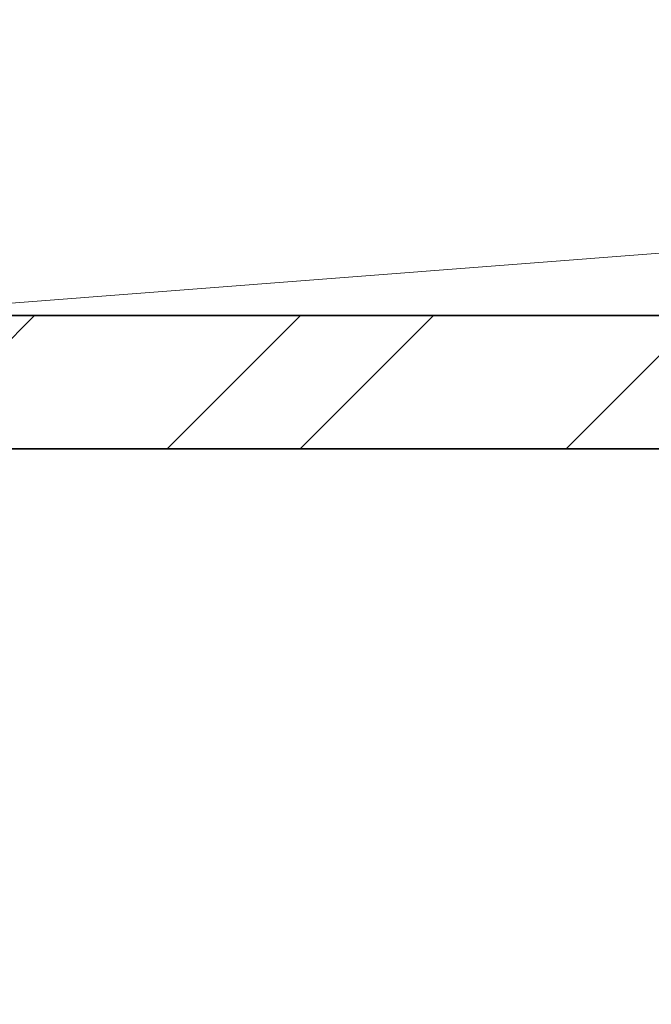
# Model space of a CAD drawing. Units: inches. Extents: x 1885 to 2748, y 783 to 2421.
# Tile 36 of 117: x 2013 to 2034, y 1501 to 1534. Entities that reach past the tile are written whole.
import ezdxf

# ---------------------------------------------------------------- set-up
doc = ezdxf.new("R2010")
doc.units = ezdxf.units.IN
doc.layers.add('A-FLOR-OPEN', color=8, linetype='Continuous', lineweight=13)
doc.layers.add('A-WALL', color=7, linetype='Continuous', lineweight=35)
doc.layers.add('A-WALL-PATT', color=85, linetype='Continuous', lineweight=13, true_color=0x58ba48)

msp = doc.modelspace()

# ---------------------------------------------------------------- hatches: boundary and pattern name
at = {"layer": 'A-WALL-PATT'}
h = msp.add_hatch(dxfattribs=at)
h.set_pattern_fill('ANSI32', color=256)
h.paths.add_polyline_path([(2007.772, 2318.006), (1980.774, 2318.006), (1980.774, 2281.215), (1985.274, 2281.215), (1985.274, 2313.506), (2007.772, 2313.506), (2007.772, 2315.756)])
h.paths.add_polyline_path([(2094.324, 2318.006), (2067.772, 2318.006), (2067.772, 2313.506), (2094.324, 2313.506), (2094.324, 2315.756)])
h.paths.add_polyline_path([(2131.367, 2315.756), (2131.367, 2318.006), (2131.189, 2318.006), (2112.609, 2318.006), (2112.609, 2313.506), (2117.274, 2313.506), (2117.274, 2255.201), (2121.774, 2255.201), (2121.774, 2313.506), (2131.367, 2313.506)])
h.paths.add_polyline_path([(2190.512, 2318.006), (2155.367, 2318.006), (2155.367, 2313.506), (2169.774, 2313.506), (2169.774, 2229.506), (2121.774, 2229.506), (2121.774, 2233.451), (2119.524, 2233.451), (2117.274, 2233.451), (2117.274, 2201.101), (2121.774, 2201.101), (2121.774, 2225.006), (2169.774, 2225.006), (2169.774, 2165.006), (2306.274, 2165.006), (2306.274, 2066.006), (2310.774, 2066.006), (2344.274, 2066.006), (2486.274, 2066.006), (2486.274, 1886.006), (2483.02, 1886.006), (2483.02, 1881.506), (2486.274, 1881.506), (2486.274, 1880.678), (2490.774, 1880.678), (2490.774, 2070.506), (2344.274, 2070.506), (2310.774, 2070.506), (2310.774, 2165.006), (2310.774, 2173.636), (2308.524, 2173.636), (2306.274, 2173.636), (2306.274, 2169.506), (2174.274, 2169.506), (2174.274, 2313.506), (2190.512, 2313.506), (2190.512, 2315.756)])
h.paths.add_polyline_path([(1985.274, 2221.215), (1980.774, 2221.215), (1980.774, 2165.006), (1992.774, 2165.006), (1992.774, 2141.927), (1997.274, 2141.927), (1997.274, 2165.006), (2117.274, 2165.006), (2117.274, 2163.126), (2121.774, 2163.126), (2121.774, 2172.734), (2119.524, 2172.734), (2117.274, 2172.734), (2117.274, 2169.506), (1985.274, 2169.506)])
h.paths.add_polyline_path([(1997.274, 2105.927), (1992.774, 2105.927), (1992.774, 2070.506), (2016.774, 2070.506), (2016.774, 2059.123), (2019.024, 2059.123), (2021.274, 2059.123), (2021.274, 2070.506), (2117.274, 2070.506), (2117.274, 2022.506), (2114.423, 2022.506), (2114.423, 2018.006), (2123.627, 2018.006), (2123.627, 2020.256), (2123.627, 2022.506), (2121.774, 2022.506), (2121.774, 2142.587), (2119.524, 2142.587), (2117.274, 2142.587), (2117.274, 2075.006), (1997.274, 2075.006)])
h.paths.add_polyline_path([(2092.029, 2020.256), (2092.029, 2022.506), (2021.274, 2022.506), (2021.274, 2035.123), (2016.774, 2035.123), (2016.774, 2018.006), (2016.774, 1978.784), (2021.274, 1978.784), (2021.274, 2018.006), (2092.029, 2018.006)])
h.paths.add_polyline_path([(2260.938, 2022.506), (2153.105, 2022.506), (2153.105, 2020.256), (2153.105, 2018.006), (2155.274, 2018.006), (2155.274, 1886.006), (2107.629, 1886.006), (2107.629, 1881.506), (2182.911, 1881.506), (2182.911, 1883.756), (2182.911, 1886.006), (2159.774, 1886.006), (2159.774, 2018.006), (2260.938, 2018.006), (2260.938, 2020.256)])
h.paths.add_polyline_path([(2047.629, 1883.756), (2047.629, 1886.006), (2021.274, 1886.006), (2021.274, 1918.784), (2019.024, 1918.784), (2016.774, 1918.784), (2016.774, 1881.506), (2047.629, 1881.506)])
h.paths.add_polyline_path([(2306.361, 1883.756), (2306.361, 1886.006), (2296.274, 1886.006), (2296.274, 1982.006), (2316.535, 1982.006), (2316.535, 1984.256), (2316.535, 1986.506), (2296.274, 1986.506), (2296.274, 2022.506), (2289.276, 2022.506), (2289.276, 2018.006), (2291.774, 2018.006), (2291.774, 1886.006), (2242.911, 1886.006), (2242.911, 1881.506), (2306.361, 1881.506)], flags=17)
h.paths.add_polyline_path([(1985.274, 1843.006), (2021.6, 1843.006), (2021.534, 1845.441), (2021.477, 1847.506), (1980.774, 1847.506), (1980.774, 1809.446), (1985.274, 1809.446)])
h.paths.add_polyline_path([(2131.482, 1845.256), (2131.482, 1847.506), (2081.534, 1847.506), (2081.534, 1843.006), (2117.274, 1843.006), (2117.274, 1784.147), (2119.524, 1784.147), (2121.774, 1784.147), (2121.774, 1843.006), (2131.482, 1843.006)])
h.paths.add_polyline_path([(2203.886, 1847.506), (2155.482, 1847.506), (2155.482, 1843.006), (2169.774, 1843.006), (2169.774, 1759.006), (2121.774, 1759.006), (2121.774, 1761.457), (2117.274, 1761.457), (2117.274, 1730.429), (2121.774, 1730.429), (2121.774, 1754.506), (2177.421, 1754.506), (2177.421, 1756.756), (2177.421, 1759.006), (2174.274, 1759.006), (2174.274, 1843.006), (2203.886, 1843.006)])
h.paths.add_polyline_path([(2335.554, 1845.256), (2335.554, 1847.506), (2239.886, 1847.506), (2239.886, 1843.006), (2306.274, 1843.006), (2306.274, 1759.006), (2199.486, 1759.006), (2199.486, 1754.506), (2310.774, 1754.506), (2310.774, 1843.006), (2335.554, 1843.006)])
h.paths.add_polyline_path([(2348.774, 2022.506), (2344.274, 2022.506), (2344.274, 1986.506), (2341.681, 1986.506), (2341.681, 1982.006), (2344.274, 1982.006), (2344.274, 1886.006), (2330.361, 1886.006), (2330.361, 1881.506), (2361.627, 1881.506), (2361.627, 1883.756), (2361.627, 1886.006), (2348.774, 1886.006)], flags=17)
h.paths.add_polyline_path([(2283.251, 2315.756), (2283.251, 2318.006), (2238.512, 2318.006), (2238.512, 2313.506), (2283.251, 2313.506)], flags=17)
h.paths.add_polyline_path([(2363.274, 2348.006), (2388.677, 2348.006), (2388.677, 2350.256), (2388.677, 2352.506), (2358.774, 2352.506), (2358.774, 2348.006), (2358.774, 2318.006), (2344.481, 2318.006), (2344.481, 2313.506), (2358.774, 2313.506), (2358.774, 2229.506), (2310.774, 2229.506), (2310.774, 2231.952), (2306.274, 2231.952), (2306.274, 2205.611), (2310.774, 2205.611), (2310.774, 2225.006), (2358.774, 2225.006), (2358.774, 2211.506), (2452.329, 2211.506), (2452.329, 2213.756), (2452.329, 2216.006), (2363.274, 2216.006), (2363.274, 2318.006)])
h.paths.add_polyline_path([(2310.774, 2313.506), (2320.481, 2313.506), (2320.481, 2315.756), (2320.481, 2318.006), (2302.728, 2318.006), (2302.728, 2313.506), (2306.274, 2313.506), (2306.274, 2251.076), (2310.774, 2251.076)], flags=17)
h.paths.add_polyline_path([(2490.774, 2352.506), (2486.274, 2352.506), (2448.677, 2352.506), (2448.677, 2348.006), (2486.274, 2348.006), (2486.274, 2318.006), (2486.274, 2216.006), (2481.78, 2216.006), (2481.78, 2211.506), (2486.274, 2211.506), (2486.274, 2165.006), (2493.289, 2165.006), (2493.289, 2167.256), (2493.289, 2169.506), (2490.774, 2169.506), (2490.774, 2313.506), (2494.429, 2313.506), (2494.429, 2318.006), (2490.774, 2318.006)])
h.paths.add_polyline_path([(2534.653, 2318.006), (2515.691, 2318.006), (2515.691, 2313.506), (2534.653, 2313.506), (2534.653, 2315.756)])
h.paths.add_polyline_path([(2618.274, 2318.006), (2594.653, 2318.006), (2594.653, 2313.506), (2613.774, 2313.506), (2613.774, 2281.706), (2618.274, 2281.706)])
h.paths.add_polyline_path([(2618.274, 2221.706), (2613.774, 2221.706), (2613.774, 2169.506), (2554.019, 2169.506), (2554.019, 2165.006), (2613.774, 2165.006), (2613.774, 2152.878), (2618.274, 2152.878)])
h.paths.add_polyline_path([(2618.274, 2128.878), (2616.024, 2128.878), (2613.774, 2128.878), (2613.774, 2117.006), (2529.774, 2117.006), (2529.774, 2165.006), (2532.848, 2165.006), (2532.848, 2169.506), (2522.867, 2169.506), (2522.867, 2165.006), (2525.274, 2165.006), (2525.274, 2117.006), (2525.274, 2112.506), (2525.274, 2108.576), (2529.774, 2108.576), (2529.774, 2112.506), (2613.774, 2112.506), (2613.774, 2080.19), (2618.274, 2080.19)])
h.paths.add_polyline_path([(2618.274, 2044.19), (2616.024, 2044.19), (2613.774, 2044.19), (2613.774, 2015.506), (2529.774, 2015.506), (2529.774, 2088.582), (2527.524, 2088.582), (2525.274, 2088.582), (2525.274, 2011.006), (2613.774, 2011.006), (2613.774, 1956.755), (2618.274, 1956.755)])
h.paths.add_polyline_path([(2618.274, 1881.506), (2618.274, 1896.755), (2613.774, 1896.755), (2613.774, 1881.506), (2613.774, 1847.506), (2592.715, 1847.506), (2592.715, 1843.006), (2613.774, 1843.006), (2613.774, 1765.006), (2613.774, 1760.506), (2609.621, 1760.506), (2609.621, 1756.006), (2613.774, 1756.006), (2613.774, 1660.006), (2608.544, 1660.006), (2608.544, 1655.506), (2613.774, 1655.506), (2613.774, 1508.158), (2618.274, 1508.158)])
h.paths.add_polyline_path([(2565.774, 1843.006), (2568.997, 1843.006), (2568.997, 1847.506), (2490.774, 1847.506), (2490.774, 1849.7), (2488.524, 1849.7), (2486.274, 1849.7), (2486.274, 1847.506), (2477.274, 1847.506), (2477.274, 1838.506), (2477.274, 1821.493), (2486.274, 1821.493), (2486.274, 1838.506), (2561.274, 1838.506), (2561.274, 1765.006), (2486.274, 1765.006), (2486.274, 1786.157), (2477.274, 1786.157), (2477.274, 1765.006), (2477.274, 1756.006), (2486.274, 1756.006), (2565.774, 1756.006), (2585.621, 1756.006), (2585.621, 1758.256), (2585.621, 1760.506), (2565.774, 1760.506), (2565.774, 1765.006)])
h.paths.add_polyline_path([(2486.274, 1651.006), (2561.274, 1651.006), (2561.274, 1567.006), (2486.274, 1567.006), (2486.274, 1591.321), (2477.274, 1591.321), (2477.274, 1567.006), (2477.274, 1558.006), (2477.274, 1555.439), (2481.774, 1555.439), (2481.774, 1558.006), (2568.653, 1558.006), (2568.653, 1560.256), (2568.653, 1562.506), (2565.774, 1562.506), (2565.774, 1655.506), (2584.544, 1655.506), (2584.544, 1657.756), (2584.544, 1660.006), (2565.774, 1660.006), (2486.274, 1660.006), (2477.274, 1660.006), (2477.274, 1651.006), (2477.274, 1632.989), (2486.274, 1632.989)])
h.paths.add_polyline_path([(2449.967, 1883.756), (2449.967, 1886.006), (2421.627, 1886.006), (2421.627, 1881.506), (2449.967, 1881.506)], flags=17)
h.paths.add_polyline_path([(2447.274, 1847.506), (2395.554, 1847.506), (2395.554, 1843.006), (2442.774, 1843.006), (2442.774, 1809.27), (2447.274, 1809.27)])
h.paths.add_polyline_path([(1985.274, 1749.446), (1980.774, 1749.446), (1980.774, 1694.504), (1985.274, 1694.504), (1985.274, 1694.506), (1986.897, 1694.506), (1986.897, 1697.78), (1986.897, 1699.006), (1985.274, 1699.006)])
h.paths.add_polyline_path([(2152.774, 1699.006), (2121.774, 1699.006), (2121.774, 1703.668), (2119.524, 1703.668), (2117.274, 1703.668), (2117.274, 1699.006), (2009.219, 1699.006), (2009.219, 1694.506), (2148.274, 1694.506), (2148.274, 1692.631), (2152.774, 1692.631)])
h.paths.add_polyline_path([(2016.274, 1694.506), (2011.774, 1694.506), (2011.774, 1558.006), (2040.806, 1558.006), (2040.806, 1560.256), (2040.806, 1562.506), (2016.274, 1562.506)])
h.paths.add_polyline_path([(2152.774, 1663.017), (2150.524, 1663.017), (2148.274, 1663.017), (2148.274, 1562.506), (2100.806, 1562.506), (2100.806, 1558.006), (2165.119, 1558.006), (2165.119, 1560.256), (2165.119, 1562.506), (2152.774, 1562.506), (2152.774, 1610.506), (2224.774, 1610.506), (2224.774, 1607.99), (2229.274, 1607.99), (2229.274, 1615.006), (2152.774, 1615.006)])
h.paths.add_polyline_path([(2238.613, 1560.256), (2238.613, 1562.506), (2229.274, 1562.506), (2229.274, 1588.756), (2227.024, 1588.763), (2224.774, 1588.771), (2224.774, 1562.506), (2189.119, 1562.506), (2189.119, 1558.006), (2238.613, 1558.006)])
h.paths.add_polyline_path([(2336.024, 1560.256), (2336.024, 1562.506), (2310.774, 1562.506), (2310.774, 1656.347), (2308.524, 1656.347), (2306.274, 1656.347), (2306.274, 1562.506), (2286.613, 1562.506), (2286.613, 1558.006), (2336.024, 1558.006)])
h.paths.add_polyline_path([(2447.274, 1690.968), (2445.024, 1690.968), (2442.774, 1690.968), (2442.774, 1687.006), (2306.274, 1687.006), (2306.274, 1680.75), (2310.774, 1680.75), (2310.774, 1682.506), (2442.774, 1682.506), (2442.774, 1562.506), (2396.024, 1562.506), (2396.024, 1558.006), (2447.274, 1558.006)])
h.paths.add_polyline_path([(2447.274, 1749.27), (2445.024, 1749.27), (2442.774, 1749.27), (2442.774, 1717.232), (2447.274, 1717.232)])
h.paths.add_polyline_path([(2044.674, 1521.756), (2044.674, 1524.006), (2007.274, 1524.006), (2007.274, 1503.49), (2009.524, 1503.49), (2011.774, 1503.49), (2011.774, 1519.506), (2044.674, 1519.506)])
h.paths.add_polyline_path([(2177.969, 1521.756), (2177.969, 1524.006), (2104.674, 1524.006), (2104.674, 1519.506), (2145.774, 1519.506), (2145.774, 1387.506), (2143.37, 1387.506), (2143.37, 1383.006), (2251.585, 1383.006), (2251.585, 1385.256), (2251.585, 1387.506), (2150.274, 1387.506), (2150.274, 1519.506), (2177.969, 1519.506)])
h.paths.add_polyline_path([(2298.704, 1524.006), (2237.969, 1524.006), (2237.969, 1519.506), (2282.274, 1519.506), (2282.274, 1387.506), (2279.683, 1387.506), (2279.683, 1383.006), (2286.774, 1383.006), (2286.774, 1419.006), (2312.451, 1419.006), (2312.451, 1421.256), (2312.451, 1423.506), (2286.774, 1423.506), (2286.774, 1519.506), (2298.704, 1519.506), (2298.704, 1521.722)], flags=17)
h.paths.add_polyline_path([(2361.897, 1521.756), (2361.897, 1524.006), (2322.704, 1524.006), (2322.704, 1519.506), (2334.774, 1519.506), (2334.774, 1423.506), (2331.93, 1423.506), (2331.93, 1419.006), (2334.774, 1419.006), (2334.774, 1387.506), (2334.774, 1383.228), (2339.274, 1383.228), (2339.274, 1387.506), (2339.274, 1519.506), (2361.897, 1519.506)], flags=17)
h.paths.add_polyline_path([(2447.274, 1521.756), (2447.274, 1524.006), (2421.897, 1524.006), (2421.897, 1519.506), (2447.274, 1519.506)], flags=17)
h.paths.add_polyline_path([(2481.774, 1529.6), (2479.524, 1529.6), (2477.274, 1529.6), (2477.274, 1524.006), (2474.489, 1524.006), (2474.489, 1519.506), (2477.274, 1519.506), (2477.274, 1334.506), (2296.774, 1334.506), (2296.774, 1240.506), (2160.274, 1240.506), (2160.274, 1180.506), (2112.274, 1180.506), (2112.274, 1207.692), (2110.024, 1207.692), (2107.774, 1207.692), (2107.774, 1171.609), (2112.274, 1171.609), (2112.274, 1176.006), (2160.274, 1176.006), (2160.274, 1092.006), (2144.221, 1092.006), (2144.221, 1087.506), (2189.497, 1087.506), (2189.497, 1089.756), (2189.497, 1092.006), (2164.774, 1092.006), (2164.774, 1236.006), (2296.774, 1236.006), (2296.774, 1231.912), (2301.274, 1231.912), (2301.274, 1330.006), (2481.774, 1330.006), (2481.774, 1387.506)])
h.paths.add_polyline_path([(2618.274, 1448.158), (2613.774, 1448.158), (2613.774, 1382.506), (2529.774, 1382.506), (2525.274, 1382.506), (2525.274, 1307.062), (2529.774, 1307.062), (2529.774, 1378.006), (2613.774, 1378.006), (2613.774, 1354.988), (2618.274, 1354.988)])
h.paths.add_polyline_path([(2618.274, 1318.988), (2613.774, 1318.988), (2613.774, 1281.006), (2529.774, 1281.006), (2529.774, 1283.786), (2527.524, 1283.786), (2525.274, 1283.786), (2525.274, 1228.506), (2516.794, 1228.506), (2516.794, 1224.006), (2533.484, 1224.006), (2533.484, 1226.256), (2533.484, 1228.506), (2529.774, 1228.506), (2529.774, 1276.506), (2613.774, 1276.506), (2613.774, 1266.02), (2618.274, 1266.02)])
h.paths.add_polyline_path([(2618.274, 1134.964), (2613.774, 1134.964), (2613.774, 1092.006), (2594.545, 1092.006), (2594.545, 1087.506), (2618.274, 1087.506)])
h.paths.add_polyline_path([(2534.545, 1092.006), (2509.765, 1092.006), (2509.765, 1087.506), (2534.545, 1087.506), (2534.545, 1089.756)])
h.paths.add_polyline_path([(2481.274, 1224.006), (2484.117, 1224.006), (2484.117, 1226.256), (2484.117, 1228.506), (2476.774, 1228.506), (2476.774, 1198.506), (2471.61, 1198.506), (2471.61, 1194.006), (2476.774, 1194.006), (2476.774, 1062.006), (2436.894, 1062.006), (2436.894, 1057.506), (2476.774, 1057.506), (2481.274, 1057.506), (2481.274, 1062.006), (2481.274, 1087.506), (2485.354, 1087.506), (2485.354, 1089.756), (2485.354, 1092.006), (2481.274, 1092.006), (2481.274, 1117.506)])
h.paths.add_polyline_path([(2439.898, 1198.506), (2349.274, 1198.506), (2349.274, 1194.006), (2349.274, 1180.506), (2301.274, 1180.506), (2301.274, 1201.896), (2299.024, 1201.896), (2296.774, 1201.896), (2296.774, 1172.335), (2299.024, 1172.335), (2301.274, 1172.335), (2301.274, 1176.006), (2349.274, 1176.006), (2349.274, 1092.006), (2334.452, 1092.006), (2334.452, 1087.506), (2349.274, 1087.506), (2349.274, 1057.506), (2353.774, 1057.506), (2376.894, 1057.506), (2376.894, 1059.756), (2376.894, 1062.006), (2353.774, 1062.006), (2353.774, 1087.506), (2353.774, 1180.506), (2353.774, 1194.006), (2439.898, 1194.006), (2439.898, 1196.256)])
h.paths.add_polyline_path([(2270.596, 1089.756), (2270.596, 1092.006), (2249.497, 1092.006), (2249.497, 1087.506), (2270.596, 1087.506)], flags=17)
h.paths.add_polyline_path([(2310.452, 1092.006), (2301.274, 1092.006), (2301.274, 1153.292), (2296.774, 1153.292), (2296.774, 1092.006), (2293.786, 1092.006), (2293.786, 1087.506), (2310.452, 1087.506), (2310.452, 1089.756)], flags=17)
h.paths.add_polyline_path([(2112.274, 1150.328), (2110.024, 1150.328), (2107.774, 1150.328), (2107.774, 1092.006), (2104.465, 1092.006), (2104.465, 1087.506), (2120.221, 1087.506), (2120.221, 1089.756), (2120.221, 1092.006), (2112.274, 1092.006)])
h.paths.add_polyline_path([(2082.172, 1092.006), (2058.144, 1092.006), (2058.144, 1087.506), (2082.172, 1087.506), (2082.172, 1089.756)])
h.paths.add_polyline_path([(1975.774, 1145.638), (1971.274, 1145.638), (1971.274, 1087.506), (1980.774, 1087.506), (1998.144, 1087.506), (1998.144, 1089.756), (1998.144, 1092.006), (1985.274, 1092.006), (1975.774, 1092.006)])
h.paths.add_polyline_path([(2112.274, 1244.385), (2110.024, 1244.385), (2107.774, 1244.385), (2107.774, 1240.506), (1992.274, 1240.506), (1992.274, 1271.008), (1987.774, 1271.008), (1987.774, 1240.506), (1980.774, 1240.506), (1975.774, 1240.506), (1971.274, 1240.506), (1971.274, 1205.638), (1975.774, 1205.638), (1975.774, 1236.006), (2107.774, 1236.006), (2107.774, 1233.444), (2112.274, 1233.444), (2112.274, 1236.006)])
h.paths.add_polyline_path([(2112.274, 1383.006), (2114.783, 1383.006), (2114.783, 1385.256), (2114.783, 1387.506), (2102.476, 1387.506), (2102.476, 1383.006), (2107.774, 1383.006), (2107.774, 1335.006), (2011.774, 1335.006), (2011.774, 1349.939), (2007.274, 1349.939), (2007.274, 1335.006), (1987.774, 1335.006), (1987.774, 1330.506), (1987.774, 1307.008), (1992.274, 1307.008), (1992.274, 1330.506), (2007.274, 1330.506), (2107.774, 1330.506), (2107.774, 1264.711), (2112.274, 1264.711)])
h.paths.add_polyline_path([(2077.857, 1387.506), (2011.774, 1387.506), (2011.774, 1390.036), (2009.524, 1390.036), (2007.274, 1390.036), (2007.274, 1373.939), (2011.774, 1373.939), (2011.774, 1383.006), (2077.857, 1383.006)])
h.paths.add_polyline_path([(2011.774, 1443.49), (2007.274, 1443.49), (2007.274, 1410.248), (2011.774, 1410.248)])

# ---------------------------------------------------------------- linework, layer by layer
at = {"layer": 'A-FLOR-OPEN'}
msp.add_line((2007.274, 1524.006), (2447.274, 1558.006), dxfattribs=at)
at = {"layer": 'A-WALL'}
for p, q in [((1980.774, 1524.006), (2044.674, 1524.006)), ((2011.774, 1519.506), (2044.674, 1519.506))]:
    msp.add_line(p, q, dxfattribs=at)

doc.saveas('drawing.dxf')
